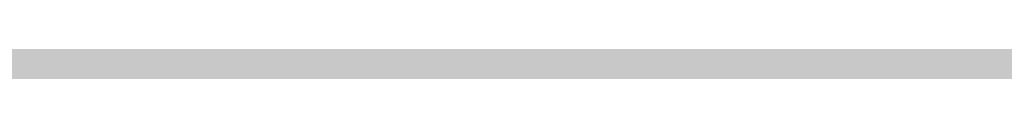
# Model space of a CAD drawing. Units: millimetres. Extents: x 0 to 2267, y 0 to 1823.
# Tile 151 of 256: x 1833.606 to 1838.83, y 1127.279 to 1127.355. Entities that reach past the tile are written whole.
import ezdxf

# ---------------------------------------------------------------- set-up
doc = ezdxf.new("R2010")
doc.units = ezdxf.units.MM
doc.header["$MEASUREMENT"] = 0
doc.layers.add('M-DIMS', color=2, linetype='Continuous', lineweight=25)
doc.layers.add('M-HATC', color=252, linetype='Continuous', lineweight=18)
doc.styles.get("Standard").update_dxf_attribs({"font": 'arial.ttf'})
doc.dimstyles.get("Standard").update_dxf_attribs({"dimtxt": 7, "dimasz": 4, "dimexe": 0.18, "dimexo": 0.0625, "dimgap": 0.09, "dimtad": 0, "dimdec": 0, "dimzin": 0, "dimdsep": 46, "dimtxsty": 'Standard', "dimcen": 0.09, "dimadec": 0, "dimazin": 0, "dimtfac": 1, "dimtdec": 0, "dimtofl": 0, "dimtmove": 0, "dimatfit": 3, "dimfxl": 1, "dimtolj": 1, "dimtzin": 0, "dimarcsym": 0})

# ---------------------------------------------------------------- blocks, each defined once
blk = doc.blocks.new('*D1')
at = {"layer": 'Defpoints', "color": 0, "transparency": 16777216}
for p in [(1593.4289, 1127.4171), (1843.4289, 1127.4171), (1843.4289, 955.6278)]:
    blk.add_point(p, dxfattribs=at)
at = {"layer": 'M-DIMS', "color": 0, "lineweight": -2, "transparency": 16777216}
for p, q in [((1593.4289, 1127.3546), (1593.4289, 955.4478)), ((1843.4289, 1127.3546), (1843.4289, 955.4478)), ((1597.4289, 955.6278), (1710.5582, 955.6278)), ((1839.4289, 955.6278), (1726.2996, 955.6278))]:
    blk.add_line(p, q, dxfattribs=at)
at = {"layer": 'M-DIMS', "color": 0, "transparency": 16777216}
for points in [[(1597.4289, 956.2944), (1597.4289, 954.9611), (1593.4289, 955.6278)], [(1839.4289, 956.2944), (1839.4289, 954.9611), (1843.4289, 955.6278)]]:
    blk.add_solid(points, dxfattribs=at)
at = {"layer": 'M-DIMS', "color": 0, "transparency": 16777216, "insert": (1718.4289, 955.6278), "char_height": 7, "attachment_point": 5}
blk.add_mtext('\\A1;250', dxfattribs=at)

msp = doc.modelspace()

# ---------------------------------------------------------------- hatches: boundary and pattern name
at = {"layer": 'M-HATC'}
h = msp.add_hatch(color=256, dxfattribs=at)
h.dxf.hatch_style = 1
h.paths.add_polyline_path([(2055.771, 1603.062), (1381.0868, 1603.062), (1381.0868, 1598.062), (2055.771, 1598.062)])
h.paths.add_polyline_path([(2055.771, 1598.062), (1381.0868, 1598.062), (1381.0868, 1593.062), (2055.771, 1593.062)])
h.paths.add_polyline_path([(2051.3074, 1536.7609), (1385.5504, 1536.7609), (1385.5504, 1526.7609), (1387.5504, 1526.7609), (1388.5366, 1525.0528), (1385.3319, 1521.2335), (1385.3319, 1521.2226), (2050.2542, 1522.7491), (2048.3212, 1525.0528), (2049.3074, 1526.7609), (2051.3074, 1526.7609)])
edge = h.paths.add_edge_path()
edge.add_arc((1847.5345, 1379.1492), 135, 222.603061, 222.890851, ccw=False)
edge.add_line((1748.1663, 1287.7656), (1683.0921, 1287.7656))
edge.add_arc((1583.7239, 1379.1492), 135, 317.109149, 317.396939, ccw=False)
edge.add_arc((1678.9686, 1290.6707), 5, 222.8909, 317.1091, ccw=False)
edge.add_arc((1774.2133, 1379.1492), 135, 222.603061, 222.890851, ccw=False)
edge.add_line((1674.8451, 1287.7656), (1609.7709, 1287.7656))
edge.add_arc((1510.4027, 1379.1492), 135, 317.109149, 317.396939, ccw=False)
edge.add_arc((1605.6474, 1290.6707), 5, 222.8909, 317.1091, ccw=False)
edge.add_arc((1700.8921, 1379.1492), 135, 222.603061, 222.890851, ccw=False)
edge.add_line((1601.5239, 1287.7656), (1536.4497, 1287.7656))
edge.add_arc((1437.0815, 1379.1492), 135, 317.109149, 317.396939, ccw=False)
edge.add_arc((1532.3262, 1290.6707), 5, 222.8909, 317.1091, ccw=False)
edge.add_arc((1627.5709, 1379.1492), 135, 222.603061, 222.890851, ccw=False)
edge.add_line((1528.2027, 1287.7656), (1505.9289, 1287.7656))
edge.add_spline(control_points=[(1505.9289, 1287.7656), (1504.2622, 1287.7656), (1504.2622, 1282.7656), (1505.9289, 1282.7656)], knot_values=[0, 0, 0, 0, 5, 5, 5, 5], degree=3, periodic=0)
edge.add_line((1505.9289, 1282.7656), (1930.9289, 1282.7656))
edge.add_spline(control_points=[(1930.9289, 1282.7656), (1932.5956, 1282.7656), (1932.5956, 1287.7656), (1930.9289, 1287.7656)], knot_values=[0, 0, 0, 0, 5, 5, 5, 5], degree=3, periodic=0)
edge.add_line((1930.9289, 1287.7656), (1903.0557, 1287.7656))
edge.add_arc((1803.6875, 1379.1492), 135, 317.109149, 317.396939, ccw=False)
edge.add_arc((1898.9322, 1290.6707), 5, 222.8909, 317.1091, ccw=False)
edge.add_arc((1994.1769, 1379.1492), 135, 222.603061, 222.890851, ccw=False)
edge.add_line((1894.8087, 1287.7656), (1829.7345, 1287.7656))
edge.add_arc((1730.3663, 1379.1492), 135, 317.109149, 317.396939, ccw=False)
edge.add_arc((1825.611, 1290.6707), 5, 222.8909, 317.1091, ccw=False)
edge.add_arc((1920.8557, 1379.1492), 135, 222.603061, 222.890851, ccw=False)
edge.add_line((1821.4875, 1287.7656), (1756.4133, 1287.7656))
edge.add_arc((1657.0451, 1379.1492), 135, 317.109149, 317.396939, ccw=False)
edge.add_arc((1752.2898, 1290.6707), 5, 222.8909, 317.1091, ccw=False)
edge = h.paths.add_edge_path()
edge.add_spline(control_points=[(1843.4289, 1227.2475), (1845.0956, 1227.2475), (1845.0956, 1232.2475), (1843.4289, 1232.2475)], knot_values=[0, 0, 0, 0, 5, 5, 5, 5], degree=3, periodic=0)
edge.add_line((1843.4289, 1232.2475), (1593.4289, 1232.2475))
edge.add_spline(control_points=[(1593.4289, 1232.2475), (1591.7622, 1232.2475), (1591.7622, 1227.2475), (1593.4289, 1227.2475)], knot_values=[0, 0, 0, 0, 5, 5, 5, 5], degree=3, periodic=0)
edge.add_line((1593.4289, 1227.2475), (1843.4289, 1227.2475))
h.paths.add_polyline_path([(1905.9289, 1127.4171), (1530.9289, 1127.4171, 0.414214), (1520.9289, 1117.4171), (1530.9289, 1117.4171), (1915.9289, 1117.4171, 0.414214)])
edge = h.paths.add_edge_path()
edge.add_arc((1397.0858, 1498.4078), 12.7299, 90.78215, 190.87871, ccw=False)
edge.add_line((1396.912, 1511.1365), (1428.0097, 1511.3488))
edge.add_line((1428.0097, 1511.3488), (1433.0097, 1511.3488))
edge.add_line((1433.0097, 1511.3488), (1434.439, 1511.3488))
edge.add_arc((1419.474, 1498.0804), 20, 41.561, 74.08211)
edge.add_line((1424.9592, 1517.3135), (1399.9351, 1517.2561))
edge.add_spline(control_points=[(1399.9307, 1517.2561), (1399.884, 1517.2131), (1399.8328, 1517.1689), (1399.7774, 1517.1236)], knot_values=[11.567499, 11.567499, 11.567499, 11.567499, 11.814249, 11.814249, 11.814249, 11.814249], degree=3, periodic=0)
edge.add_spline(control_points=[(1399.6328, 1517.0099), (1399.5831, 1516.9721), (1399.5307, 1516.9338), (1399.4759, 1516.8947)], knot_values=[11.167718, 11.167718, 11.167718, 11.167718, 11.365188, 11.365188, 11.365188, 11.365188], degree=3, periodic=0)
edge.add_spline(control_points=[(1399.3398, 1516.8001), (1399.1514, 1516.6719), (1398.9384, 1516.5377), (1398.704, 1516.3994)], knot_values=[10.376405, 10.376405, 10.376405, 10.376405, 11.00994, 11.00994, 11.00994, 11.00994], degree=3, periodic=0)
edge.add_spline(control_points=[(1398.6572, 1516.3719), (1398.5789, 1516.326), (1398.4983, 1516.2797), (1398.4155, 1516.2331)], knot_values=[10.125175, 10.125175, 10.125175, 10.125175, 10.334406, 10.334406, 10.334406, 10.334406], degree=3, periodic=0)
edge.add_spline(control_points=[(1398.2642, 1516.1487), (1398.196, 1516.1111), (1398.1263, 1516.0732), (1398.0555, 1516.0351)], knot_values=[9.832246, 9.832246, 9.832246, 9.832246, 9.999658, 9.999658, 9.999658, 9.999658], degree=3, periodic=0)
edge.add_spline(control_points=[(1397.9987, 1516.0048), (1397.7312, 1515.8621), (1397.446, 1515.7171), (1397.1466, 1515.5714)], knot_values=[9.161808, 9.161808, 9.161808, 9.161808, 9.787769, 9.787769, 9.787769, 9.787769], degree=3, periodic=0)
edge.add_spline(control_points=[(1397.1466, 1515.5714), (1396.8418, 1515.423), (1396.5222, 1515.274), (1396.1914, 1515.1262)], knot_values=[8.524455, 8.524455, 8.524455, 8.524455, 9.161808, 9.161808, 9.161808, 9.161808], degree=3, periodic=0)
edge.add_spline(control_points=[(1396.0777, 1515.0756), (1395.9854, 1515.0348), (1395.8922, 1514.994), (1395.7983, 1514.9534)], knot_values=[8.275193, 8.275193, 8.275193, 8.275193, 8.451726, 8.451726, 8.451726, 8.451726], degree=3, periodic=0)
edge.add_spline(control_points=[(1395.6018, 1514.8691), (1395.4997, 1514.8257), (1395.3968, 1514.7824), (1395.2932, 1514.7394)], knot_values=[7.962917, 7.962917, 7.962917, 7.962917, 8.152764, 8.152764, 8.152764, 8.152764], degree=3, periodic=0)
edge.add_spline(control_points=[(1395.2116, 1514.7057), (1394.8278, 1514.5475), (1394.4345, 1514.3929), (1394.0364, 1514.2442)], knot_values=[7.21254, 7.21254, 7.21254, 7.21254, 7.913148, 7.913148, 7.913148, 7.913148], degree=3, periodic=0)
edge.add_spline(control_points=[(1394.0364, 1514.2442), (1393.7076, 1514.1214), (1393.3754, 1514.0027), (1393.0427, 1513.8895)], knot_values=[6.633733, 6.633733, 6.633733, 6.633733, 7.21254, 7.21254, 7.21254, 7.21254], degree=3, periodic=0)
edge.add_spline(control_points=[(1392.8214, 1513.815), (1392.7198, 1513.7812), (1392.6181, 1513.7479), (1392.5166, 1513.7152)], knot_values=[6.328796, 6.328796, 6.328796, 6.328796, 6.505493, 6.505493, 6.505493, 6.505493], degree=3, periodic=0)
edge.add_spline(control_points=[(1392.5166, 1513.7152), (1392.3187, 1513.6515), (1392.1212, 1513.59), (1391.9244, 1513.531)], knot_values=[5.984605, 5.984605, 5.984605, 5.984605, 6.328796, 6.328796, 6.328796, 6.328796], degree=3, periodic=0)
edge.add_spline(control_points=[(1391.7915, 1513.4915), (1391.3122, 1513.3501), (1390.8384, 1513.2239), (1390.3784, 1513.1171)], knot_values=[5.066697, 5.066697, 5.066697, 5.066697, 5.907055, 5.907055, 5.907055, 5.907055], degree=3, periodic=0)
edge.add_spline(control_points=[(1390.3784, 1513.1171), (1390.1797, 1513.071), (1389.9836, 1513.0284), (1389.7907, 1512.9899)], knot_values=[4.70367, 4.70367, 4.70367, 4.70367, 5.066695, 5.066695, 5.066695, 5.066695], degree=3, periodic=0)
edge.add_spline(control_points=[(1389.422, 1512.9204), (1389.2459, 1512.8892), (1389.0729, 1512.8617), (1388.9036, 1512.8381)], knot_values=[4.130571, 4.130571, 4.130571, 4.130571, 4.469816, 4.469816, 4.469816, 4.469816], degree=3, periodic=0)
edge.add_spline(control_points=[(1388.9036, 1512.8381), (1388.591, 1512.7946), (1388.2911, 1512.7644), (1388.0071, 1512.7494)], knot_values=[3.504031, 3.504031, 3.504031, 3.504031, 4.130571, 4.130571, 4.130571, 4.130571], degree=3, periodic=0)
edge.add_spline(control_points=[(1387.9356, 1512.7459), (1387.8538, 1512.7423), (1387.7733, 1512.74), (1387.6944, 1512.739)], knot_values=[3.268866, 3.268866, 3.268866, 3.268866, 3.451164, 3.451164, 3.451164, 3.451164], degree=3, periodic=0)
edge.add_spline(control_points=[(1387.3351, 1512.7443), (1387.2076, 1512.7499), (1387.0847, 1512.7597), (1386.967, 1512.7739)], knot_values=[2.670686, 2.670686, 2.670686, 2.670686, 2.984, 2.984, 2.984, 2.984], degree=3, periodic=0)
edge.add_spline(control_points=[(1386.8327, 1512.7922), (1386.8209, 1512.7941), (1386.8092, 1512.7959), (1386.7975, 1512.7979)], knot_values=[2.516981, 2.516981, 2.516981, 2.516981, 2.549528, 2.549528, 2.549528, 2.549528], degree=3, periodic=0)
edge.add_spline(control_points=[(1386.4526, 1512.8735), (1386.4257, 1512.881), (1386.3993, 1512.889), (1386.3733, 1512.8972)], knot_values=[2.095869, 2.095869, 2.095869, 2.095869, 2.17941, 2.17941, 2.17941, 2.17941], degree=3, periodic=0)
edge.add_spline(control_points=[(1386.0691, 1513.0189), (1386.0634, 1513.0217), (1386.0577, 1513.0246), (1386.052, 1513.0275)], knot_values=[1.72453, 1.72453, 1.72453, 1.72453, 1.745933, 1.745933, 1.745933, 1.745933], degree=3, periodic=0)
edge.add_arc((1399.474, 1498.0804), 20, 131.82432, 180)
edge.add_arc((1630.3336, 1505.5484), 250.9708, 181.705176, 236.427975)
edge.add_arc((1605.3399, 1483.3044), 218.7822, 238.660829, 243.34961)
edge.add_arc((1647.0911, 1510.3592), 262.8986, 183.129836, 237.853442, ccw=False)
h.paths.add_polyline_path([(1406.5369, 1391.9644, 0.149382), (1491.5506, 1296.4418, -0.129517)], flags=17)
edge = h.paths.add_edge_path()
edge.add_arc((2037.3838, 1498.0804), 20, 0, 48.26587)
edge.add_spline(control_points=[(2050.6973, 1513.0052), (2050.6512, 1512.9847), (2050.6034, 1512.9655), (2050.5539, 1512.9477)], knot_values=[1.835652, 1.835652, 1.835652, 1.835652, 2.000781, 2.000781, 2.000781, 2.000781], degree=3, periodic=0)
edge.add_spline(control_points=[(2050.4616, 1512.9166), (2050.479, 1512.9221), (2050.4963, 1512.9277), (2050.5133, 1512.9335)], knot_values=[2.045477, 2.045477, 2.045477, 2.045477, 2.101389, 2.101389, 2.101389, 2.101389], degree=3, periodic=0)
edge.add_spline(control_points=[(2050.129, 1512.8342), (2050.1984, 1512.8473), (2050.2657, 1512.8623), (2050.3308, 1512.8792)], knot_values=[2.237629, 2.237629, 2.237629, 2.237629, 2.435841, 2.435841, 2.435841, 2.435841], degree=3, periodic=0)
edge.add_spline(control_points=[(2050.0946, 1512.8278), (2050.1061, 1512.8299), (2050.1176, 1512.832), (2050.129, 1512.8342)], knot_values=[2.435841, 2.435841, 2.435841, 2.435841, 2.468321, 2.468321, 2.468321, 2.468321], degree=3, periodic=0)
edge.add_spline(control_points=[(2049.7843, 1512.7851), (2049.8552, 1512.7922), (2049.9243, 1512.8008), (2049.9917, 1512.8109)], knot_values=[2.563852, 2.563852, 2.563852, 2.563852, 2.748541, 2.748541, 2.748541, 2.748541], degree=3, periodic=0)
edge.add_spline(control_points=[(2049.4052, 1512.7617), (2049.5364, 1512.7653), (2049.6629, 1512.773), (2049.7843, 1512.7851)], knot_values=[2.748541, 2.748541, 2.748541, 2.748541, 3.064882, 3.064882, 3.064882, 3.064882], degree=3, periodic=0)
edge.add_spline(control_points=[(2049.1698, 1512.7597), (2049.2336, 1512.7591), (2049.2965, 1512.7594), (2049.3584, 1512.7606)], knot_values=[3.102309, 3.102309, 3.102309, 3.102309, 3.2503, 3.2503, 3.2503, 3.2503], degree=3, periodic=0)
edge.add_spline(control_points=[(2048.8573, 1512.7691), (2048.9638, 1512.7638), (2049.068, 1512.7606), (2049.1698, 1512.7597)], knot_values=[3.2503, 3.2503, 3.2503, 3.2503, 3.486069, 3.486069, 3.486069, 3.486069], degree=3, periodic=0)
edge.add_spline(control_points=[(2048.6924, 1512.7789), (2048.3729, 1512.8009), (2048.0345, 1512.8411), (2047.6817, 1512.897)], knot_values=[3.606429, 3.606429, 3.606429, 3.606429, 4.2989, 4.2989, 4.2989, 4.2989], degree=3, periodic=0)
edge.add_spline(control_points=[(2047.6817, 1512.897), (2047.5458, 1512.9185), (2047.4077, 1512.9424), (2047.2678, 1512.9685)], knot_values=[4.2989, 4.2989, 4.2989, 4.2989, 4.565769, 4.565769, 4.565769, 4.565769], degree=3, periodic=0)
edge.add_spline(control_points=[(2047.2678, 1512.9685), (2047.1449, 1512.9914), (2047.0207, 1513.016), (2046.8951, 1513.0422)], knot_values=[4.565769, 4.565769, 4.565769, 4.565769, 4.799971, 4.799971, 4.799971, 4.799971], degree=3, periodic=0)
edge.add_spline(control_points=[(2046.8951, 1513.0422), (2046.5286, 1513.1188), (2046.1513, 1513.209), (2045.7676, 1513.3107)], knot_values=[4.799971, 4.799971, 4.799971, 4.799971, 5.483718, 5.483718, 5.483718, 5.483718], degree=3, periodic=0)
edge.add_spline(control_points=[(2045.7676, 1513.3107), (2045.3724, 1513.4154), (2044.9704, 1513.5322), (2044.5662, 1513.6588)], knot_values=[5.483718, 5.483718, 5.483718, 5.483718, 6.187866, 6.187866, 6.187866, 6.187866], degree=3, periodic=0)
edge.add_spline(control_points=[(2044.5662, 1513.6588), (2044.4149, 1513.7061), (2044.2633, 1513.7549), (2044.1116, 1513.8048)], knot_values=[6.187866, 6.187866, 6.187866, 6.187866, 6.451551, 6.451551, 6.451551, 6.451551], degree=3, periodic=0)
edge.add_spline(control_points=[(2044.1116, 1513.8048), (2043.9967, 1513.8427), (2043.8817, 1513.8813), (2043.7668, 1513.9205)], knot_values=[6.451551, 6.451551, 6.451551, 6.451551, 6.651434, 6.651434, 6.651434, 6.651434], degree=3, periodic=0)
edge.add_spline(control_points=[(2043.7668, 1513.9205), (2043.3716, 1514.0554), (2042.9774, 1514.1979), (2042.5886, 1514.3458)], knot_values=[6.651434, 6.651434, 6.651434, 6.651434, 7.338879, 7.338879, 7.338879, 7.338879], degree=3, periodic=0)
edge.add_spline(control_points=[(2042.5886, 1514.3458), (2042.1643, 1514.5071), (2041.7465, 1514.6749), (2041.3409, 1514.846)], knot_values=[7.338879, 7.338879, 7.338879, 7.338879, 8.089209, 8.089209, 8.089209, 8.089209], degree=3, periodic=0)
edge.add_spline(control_points=[(2041.3409, 1514.846), (2041.1028, 1514.9465), (2040.869, 1515.0481), (2040.6405, 1515.1502)], knot_values=[8.089209, 8.089209, 8.089209, 8.089209, 8.529587, 8.529587, 8.529587, 8.529587], degree=3, periodic=0)
edge.add_spline(control_points=[(2040.51, 1515.2089), (2040.0824, 1515.4022), (2039.6747, 1515.5971), (2039.295, 1515.7894)], knot_values=[8.613818, 8.613818, 8.613818, 8.613818, 9.44571, 9.44571, 9.44571, 9.44571], degree=3, periodic=0)
edge.add_spline(control_points=[(2039.295, 1515.7894), (2039.0618, 1515.9075), (2038.8391, 1516.0246), (2038.6288, 1516.1398)], knot_values=[9.44571, 9.44571, 9.44571, 9.44571, 9.956404, 9.956404, 9.956404, 9.956404], degree=3, periodic=0)
edge.add_spline(control_points=[(2038.6288, 1516.1398), (2038.5187, 1516.2001), (2038.4121, 1516.2598), (2038.309, 1516.3189)], knot_values=[9.956404, 9.956404, 9.956404, 9.956404, 10.223542, 10.223542, 10.223542, 10.223542], degree=3, periodic=0)
edge.add_spline(control_points=[(2038.309, 1516.3189), (2038.2138, 1516.3735), (2038.1216, 1516.4276), (2038.0328, 1516.481)], knot_values=[10.223542, 10.223542, 10.223542, 10.223542, 10.47051, 10.47051, 10.47051, 10.47051], degree=3, periodic=0)
edge.add_spline(control_points=[(2038.0328, 1516.481), (2037.7855, 1516.6296), (2037.5639, 1516.773), (2037.3722, 1516.909)], knot_values=[10.47051, 10.47051, 10.47051, 10.47051, 11.15767, 11.15767, 11.15767, 11.15767], degree=3, periodic=0)
edge.add_spline(control_points=[(2037.3722, 1516.909), (2037.2789, 1516.9752), (2037.1927, 1517.0396), (2037.1142, 1517.102)], knot_values=[11.15767, 11.15767, 11.15767, 11.15767, 11.49227, 11.49227, 11.49227, 11.49227], degree=3, periodic=0)
edge.add_spline(control_points=[(2036.8564, 1517.3259), (2036.9148, 1517.2692), (2036.9814, 1517.2103), (2037.0557, 1517.1492)], knot_values=[11.577341, 11.577341, 11.577341, 11.577341, 11.91035, 11.91035, 11.91035, 11.91035], degree=3, periodic=0)
edge.add_spline(control_points=[(2036.8074, 1517.3748), (2036.823, 1517.3587), (2036.8393, 1517.3424), (2036.8564, 1517.3259)], knot_values=[11.91035, 11.91035, 11.91035, 11.91035, 12.007402, 12.007402, 12.007402, 12.007402], degree=3, periodic=0)
edge.add_spline(control_points=[(2036.7017, 1517.494), (2036.7104, 1517.483), (2036.7196, 1517.4719), (2036.7291, 1517.4606)], knot_values=[12.184155, 12.184155, 12.184155, 12.184155, 12.255409, 12.255409, 12.255409, 12.255409], degree=3, periodic=0)
edge.add_spline(control_points=[(2036.6159, 1517.6205), (2036.62, 1517.613), (2036.6243, 1517.6055), (2036.6289, 1517.5979)], knot_values=[12.487913, 12.487913, 12.487913, 12.487913, 12.541035, 12.541035, 12.541035, 12.541035], degree=3, periodic=0)
edge.add_spline(control_points=[(2036.5635, 1517.786), (2036.5637, 1517.7794), (2036.5642, 1517.7726), (2036.565, 1517.7658)], knot_values=[12.911761, 12.911761, 12.911761, 12.911761, 12.968286, 12.968286, 12.968286, 12.968286], degree=3, periodic=0)
edge.add_spline(control_points=[(2036.6166, 1517.9304), (2036.6125, 1517.9259), (2036.6086, 1517.9212), (2036.6049, 1517.9165)], knot_values=[13.382527, 13.382527, 13.382527, 13.382527, 13.433791, 13.433791, 13.433791, 13.433791], degree=3, periodic=0)
edge.add_spline(control_points=[(2036.749, 1518.017), (2036.7361, 1518.0116), (2036.7239, 1518.006), (2036.7124, 1518.0002)], knot_values=[13.726299, 13.726299, 13.726299, 13.726299, 13.809928, 13.809928, 13.809928, 13.809928], degree=3, periodic=0)
edge.add_spline(control_points=[(2036.8604, 1518.0528), (2036.8386, 1518.0474), (2036.8181, 1518.0416), (2036.7988, 1518.0353)], knot_values=[13.910887, 13.910887, 13.910887, 13.910887, 14.02153, 14.02153, 14.02153, 14.02153], degree=3, periodic=0)
edge.add_line((2036.9639, 1518.0804), (2032.3838, 1518.0804))
edge.add_line((2032.3838, 1518.0804), (2027.3838, 1518.0804))
edge.add_line((2027.3838, 1518.0804), (2022.3838, 1518.0804))
edge.add_line((2022.3838, 1518.0804), (2017.3838, 1518.0804))
edge.add_arc((2017.3838, 1498.0804), 20, 90, 138.439)
edge.add_line((2002.4188, 1511.3488), (2003.8481, 1511.3488))
edge.add_line((2003.8481, 1511.3488), (2008.8481, 1511.3488))
edge.add_line((2008.8481, 1511.3488), (2039.772, 1511.1377))
edge.add_arc((2039.772, 1498.4078), 12.7299, -10.87871, 90, ccw=False)
edge.add_arc((1789.7668, 1510.3592), 262.8986, 302.146558, 356.870164, ccw=False)
edge.add_arc((1831.5179, 1483.3044), 218.7822, 296.65039, 301.339171)
edge.add_arc((1806.5242, 1505.5484), 250.9708, 303.572025, 358.294824)
h.paths.add_polyline_path([(2030.321, 1391.9644, -0.129517), (1945.3072, 1296.4418, 0.149382)], flags=17)
edge = h.paths.add_edge_path()
edge.add_spline(control_points=[(2037.2464, 1518.0821), (2037.2898, 1518.081), (2037.3355, 1518.0804), (2037.3838, 1518.0804)], knot_values=[0.000012, 0.000012, 0.000012, 0.000012, 0.144754, 0.144754, 0.144754, 0.144754], degree=3, periodic=0)
edge.add_line((2037.3357, 1518.0804), (2037.0096, 1518.0804))
edge.add_spline(control_points=[(2037.0096, 1518.0804), (2036.9822, 1518.0768), (2036.956, 1518.0727), (2036.9312, 1518.0681)], knot_values=[14.13465, 14.13465, 14.13465, 14.13465, 14.247197, 14.247197, 14.247197, 14.247197], degree=3, periodic=0)
edge.add_spline(control_points=[(2036.9312, 1518.0681), (2036.9276, 1518.0674), (2036.9241, 1518.0667), (2036.9205, 1518.0661)], knot_values=[14.118315, 14.118315, 14.118315, 14.118315, 14.13465, 14.13465, 14.13465, 14.13465], degree=3, periodic=0)
edge.add_spline(control_points=[(2036.9205, 1518.0661), (2036.9118, 1518.0644), (2036.9032, 1518.0626), (2036.8948, 1518.0608)], knot_values=[14.078086, 14.078086, 14.078086, 14.078086, 14.118315, 14.118315, 14.118315, 14.118315], degree=3, periodic=0)
edge.add_spline(control_points=[(2036.8948, 1518.0608), (2036.883, 1518.0583), (2036.8716, 1518.0556), (2036.8604, 1518.0528)], knot_values=[14.02153, 14.02153, 14.02153, 14.02153, 14.078086, 14.078086, 14.078086, 14.078086], degree=3, periodic=0)
edge.add_spline(control_points=[(2036.8604, 1518.0528), (2036.8386, 1518.0474), (2036.8181, 1518.0416), (2036.7988, 1518.0353)], knot_values=[13.910887, 13.910887, 13.910887, 13.910887, 14.02153, 14.02153, 14.02153, 14.02153], degree=3, periodic=0)
edge.add_spline(control_points=[(2036.7988, 1518.0353), (2036.7981, 1518.035), (2036.7974, 1518.0348), (2036.7967, 1518.0346)], knot_values=[13.906906, 13.906906, 13.906906, 13.906906, 13.910887, 13.910887, 13.910887, 13.910887], degree=3, periodic=0)
edge.add_spline(control_points=[(2036.7967, 1518.0346), (2036.7882, 1518.0318), (2036.7799, 1518.0289), (2036.7719, 1518.0259)], knot_values=[13.857826, 13.857826, 13.857826, 13.857826, 13.906906, 13.906906, 13.906906, 13.906906], degree=3, periodic=0)
edge.add_spline(control_points=[(2036.7719, 1518.0259), (2036.764, 1518.023), (2036.7564, 1518.02), (2036.749, 1518.017)], knot_values=[13.809928, 13.809928, 13.809928, 13.809928, 13.857826, 13.857826, 13.857826, 13.857826], degree=3, periodic=0)
edge.add_spline(control_points=[(2036.749, 1518.017), (2036.7361, 1518.0116), (2036.7239, 1518.006), (2036.7124, 1518.0002)], knot_values=[13.726299, 13.726299, 13.726299, 13.726299, 13.809928, 13.809928, 13.809928, 13.809928], degree=3, periodic=0)
edge.add_spline(control_points=[(2036.7124, 1518.0002), (2036.7121, 1518), (2036.7118, 1517.9999), (2036.7115, 1517.9997)], knot_values=[13.723993, 13.723993, 13.723993, 13.723993, 13.726299, 13.726299, 13.726299, 13.726299], degree=3, periodic=0)
edge.add_spline(control_points=[(2036.7115, 1517.9997), (2036.7063, 1517.9971), (2036.7013, 1517.9944), (2036.6965, 1517.9917)], knot_values=[13.686536, 13.686536, 13.686536, 13.686536, 13.723993, 13.723993, 13.723993, 13.723993], degree=3, periodic=0)
edge.add_spline(control_points=[(2036.6965, 1517.9917), (2036.6919, 1517.9891), (2036.6874, 1517.9865), (2036.6831, 1517.9839)], knot_values=[13.651251, 13.651251, 13.651251, 13.651251, 13.686536, 13.686536, 13.686536, 13.686536], degree=3, periodic=0)
edge.add_spline(control_points=[(2036.6831, 1517.9839), (2036.6764, 1517.9798), (2036.67, 1517.9757), (2036.6639, 1517.9714)], knot_values=[13.596804, 13.596804, 13.596804, 13.596804, 13.651251, 13.651251, 13.651251, 13.651251], degree=3, periodic=0)
edge.add_spline(control_points=[(2036.6639, 1517.9714), (2036.6636, 1517.9712), (2036.6633, 1517.9709), (2036.6629, 1517.9707)], knot_values=[13.593956, 13.593956, 13.593956, 13.593956, 13.596804, 13.596804, 13.596804, 13.596804], degree=3, periodic=0)
edge.add_spline(control_points=[(2036.6629, 1517.9707), (2036.6603, 1517.9689), (2036.6577, 1517.967), (2036.6552, 1517.9651)], knot_values=[13.570322, 13.570322, 13.570322, 13.570322, 13.593956, 13.593956, 13.593956, 13.593956], degree=3, periodic=0)
edge.add_spline(control_points=[(2036.6552, 1517.9651), (2036.6525, 1517.9631), (2036.6499, 1517.9611), (2036.6474, 1517.9591)], knot_values=[13.545477, 13.545477, 13.545477, 13.545477, 13.570322, 13.570322, 13.570322, 13.570322], degree=3, periodic=0)
edge.add_spline(control_points=[(2036.6474, 1517.9591), (2036.6472, 1517.9589), (2036.6471, 1517.9588), (2036.6469, 1517.9587)], knot_values=[13.543931, 13.543931, 13.543931, 13.543931, 13.545477, 13.545477, 13.545477, 13.545477], degree=3, periodic=0)
edge.add_spline(control_points=[(2036.6469, 1517.9587), (2036.6412, 1517.9541), (2036.6358, 1517.9494), (2036.6307, 1517.9447)], knot_values=[13.488237, 13.488237, 13.488237, 13.488237, 13.543931, 13.543931, 13.543931, 13.543931], degree=3, periodic=0)
edge.add_spline(control_points=[(2036.6307, 1517.9447), (2036.6282, 1517.9423), (2036.6257, 1517.9399), (2036.6233, 1517.9374)], knot_values=[13.460307, 13.460307, 13.460307, 13.460307, 13.488237, 13.488237, 13.488237, 13.488237], degree=3, periodic=0)
edge.add_spline(control_points=[(2036.6233, 1517.9374), (2036.6215, 1517.9356), (2036.6198, 1517.9338), (2036.6181, 1517.932)], knot_values=[13.439712, 13.439712, 13.439712, 13.439712, 13.460307, 13.460307, 13.460307, 13.460307], degree=3, periodic=0)
edge.add_spline(control_points=[(2036.6181, 1517.932), (2036.6176, 1517.9315), (2036.6171, 1517.9309), (2036.6166, 1517.9304)], knot_values=[13.433791, 13.433791, 13.433791, 13.433791, 13.439712, 13.439712, 13.439712, 13.439712], degree=3, periodic=0)
edge.add_spline(control_points=[(2036.6166, 1517.9304), (2036.6125, 1517.9259), (2036.6086, 1517.9212), (2036.6049, 1517.9165)], knot_values=[13.382527, 13.382527, 13.382527, 13.382527, 13.433791, 13.433791, 13.433791, 13.433791], degree=3, periodic=0)
edge.add_spline(control_points=[(2036.6049, 1517.9165), (2036.6026, 1517.9135), (2036.6004, 1517.9104), (2036.5982, 1517.9074)], knot_values=[13.350017, 13.350017, 13.350017, 13.350017, 13.382527, 13.382527, 13.382527, 13.382527], degree=3, periodic=0)
edge.add_spline(control_points=[(2036.5982, 1517.9074), (2036.5972, 1517.9059), (2036.5962, 1517.9043), (2036.5952, 1517.9028)], knot_values=[13.333922, 13.333922, 13.333922, 13.333922, 13.350017, 13.350017, 13.350017, 13.350017], degree=3, periodic=0)
edge.add_spline(control_points=[(2036.5952, 1517.9028), (2036.5945, 1517.9018), (2036.5939, 1517.9009), (2036.5933, 1517.8999)], knot_values=[13.323828, 13.323828, 13.323828, 13.323828, 13.333922, 13.333922, 13.333922, 13.333922], degree=3, periodic=0)
edge.add_spline(control_points=[(2036.5933, 1517.8999), (2036.5905, 1517.8955), (2036.5879, 1517.8909), (2036.5855, 1517.8864)], knot_values=[13.277545, 13.277545, 13.277545, 13.277545, 13.323828, 13.323828, 13.323828, 13.323828], degree=3, periodic=0)
edge.add_spline(control_points=[(2036.5855, 1517.8864), (2036.5836, 1517.8827), (2036.5817, 1517.8789), (2036.5801, 1517.8751)], knot_values=[13.240119, 13.240119, 13.240119, 13.240119, 13.277545, 13.277545, 13.277545, 13.277545], degree=3, periodic=0)
edge.add_spline(control_points=[(2036.5801, 1517.8751), (2036.5795, 1517.8739), (2036.579, 1517.8727), (2036.5785, 1517.8715)], knot_values=[13.228211, 13.228211, 13.228211, 13.228211, 13.240119, 13.240119, 13.240119, 13.240119], degree=3, periodic=0)
edge.add_spline(control_points=[(2036.5785, 1517.8715), (2036.578, 1517.8702), (2036.5774, 1517.869), (2036.5769, 1517.8677)], knot_values=[13.215717, 13.215717, 13.215717, 13.215717, 13.228211, 13.228211, 13.228211, 13.228211], degree=3, periodic=0)
edge.add_spline(control_points=[(2036.5769, 1517.8677), (2036.5755, 1517.864), (2036.5741, 1517.8603), (2036.5729, 1517.8565)], knot_values=[13.179847, 13.179847, 13.179847, 13.179847, 13.215717, 13.215717, 13.215717, 13.215717], degree=3, periodic=0)
edge.add_spline(control_points=[(2036.5729, 1517.8565), (2036.5713, 1517.8515), (2036.5699, 1517.8464), (2036.5687, 1517.8413)], knot_values=[13.132017, 13.132017, 13.132017, 13.132017, 13.179847, 13.179847, 13.179847, 13.179847], degree=3, periodic=0)
edge.add_spline(control_points=[(2036.5687, 1517.8413), (2036.5684, 1517.8402), (2036.5682, 1517.8392), (2036.568, 1517.8382)], knot_values=[13.122482, 13.122482, 13.122482, 13.122482, 13.132017, 13.132017, 13.132017, 13.132017], degree=3, periodic=0)
edge.add_spline(control_points=[(2036.568, 1517.8382), (2036.5676, 1517.8363), (2036.5672, 1517.8345), (2036.5669, 1517.8327)], knot_values=[13.105592, 13.105592, 13.105592, 13.105592, 13.122482, 13.122482, 13.122482, 13.122482], degree=3, periodic=0)
edge.add_spline(control_points=[(2036.5669, 1517.8327), (2036.5662, 1517.8292), (2036.5657, 1517.8257), (2036.5652, 1517.8222)], knot_values=[13.074063, 13.074063, 13.074063, 13.074063, 13.105592, 13.105592, 13.105592, 13.105592], degree=3, periodic=0)
edge.add_spline(control_points=[(2036.5652, 1517.8222), (2036.5652, 1517.8222), (2036.5652, 1517.8222), (2036.5652, 1517.8222)], knot_values=[13.074043, 13.074043, 13.074043, 13.074043, 13.074063, 13.074063, 13.074063, 13.074063], degree=3, periodic=0)
edge.add_spline(control_points=[(2036.5652, 1517.8222), (2036.5644, 1517.8164), (2036.5639, 1517.8106), (2036.5636, 1517.8046)], knot_values=[13.021884, 13.021884, 13.021884, 13.021884, 13.074043, 13.074043, 13.074043, 13.074043], degree=3, periodic=0)
edge.add_spline(control_points=[(2036.5636, 1517.8046), (2036.5636, 1517.804), (2036.5636, 1517.8034), (2036.5635, 1517.8028)], knot_values=[13.01674, 13.01674, 13.01674, 13.01674, 13.021884, 13.021884, 13.021884, 13.021884], degree=3, periodic=0)
edge.add_spline(control_points=[(2036.5635, 1517.8028), (2036.5634, 1517.8005), (2036.5634, 1517.7982), (2036.5634, 1517.7958)], knot_values=[12.996438, 12.996438, 12.996438, 12.996438, 13.01674, 13.01674, 13.01674, 13.01674], degree=3, periodic=0)
edge.add_spline(control_points=[(2036.5634, 1517.7958), (2036.5633, 1517.7926), (2036.5634, 1517.7893), (2036.5635, 1517.786)], knot_values=[12.968286, 12.968286, 12.968286, 12.968286, 12.996438, 12.996438, 12.996438, 12.996438], degree=3, periodic=0)
edge.add_spline(control_points=[(2036.5635, 1517.786), (2036.5637, 1517.7794), (2036.5642, 1517.7726), (2036.565, 1517.7658)], knot_values=[12.911761, 12.911761, 12.911761, 12.911761, 12.968286, 12.968286, 12.968286, 12.968286], degree=3, periodic=0)
edge.add_spline(control_points=[(2036.565, 1517.7658), (2036.565, 1517.7657), (2036.565, 1517.7656), (2036.565, 1517.7656)], knot_values=[12.911017, 12.911017, 12.911017, 12.911017, 12.911761, 12.911761, 12.911761, 12.911761], degree=3, periodic=0)
edge.add_spline(control_points=[(2036.565, 1517.7656), (2036.5654, 1517.7625), (2036.5658, 1517.7593), (2036.5663, 1517.7562)], knot_values=[12.88528, 12.88528, 12.88528, 12.88528, 12.911017, 12.911017, 12.911017, 12.911017], degree=3, periodic=0)
edge.add_spline(control_points=[(2036.5663, 1517.7562), (2036.5667, 1517.7534), (2036.5672, 1517.7506), (2036.5677, 1517.7478)], knot_values=[12.862519, 12.862519, 12.862519, 12.862519, 12.88528, 12.88528, 12.88528, 12.88528], degree=3, periodic=0)
edge.add_spline(control_points=[(2036.5677, 1517.7478), (2036.5678, 1517.7474), (2036.5679, 1517.7469), (2036.568, 1517.7465)], knot_values=[12.858885, 12.858885, 12.858885, 12.858885, 12.862519, 12.862519, 12.862519, 12.862519], degree=3, periodic=0)
edge.add_spline(control_points=[(2036.568, 1517.7465), (2036.5692, 1517.7399), (2036.5707, 1517.7332), (2036.5724, 1517.7264)], knot_values=[12.8053, 12.8053, 12.8053, 12.8053, 12.858885, 12.858885, 12.858885, 12.858885], degree=3, periodic=0)
edge.add_spline(control_points=[(2036.5724, 1517.7264), (2036.5734, 1517.7226), (2036.5745, 1517.7187), (2036.5756, 1517.7149)], knot_values=[12.775176, 12.775176, 12.775176, 12.775176, 12.8053, 12.8053, 12.8053, 12.8053], degree=3, periodic=0)
edge.add_spline(control_points=[(2036.5756, 1517.7149), (2036.5763, 1517.7125), (2036.577, 1517.7102), (2036.5778, 1517.7078)], knot_values=[12.756759, 12.756759, 12.756759, 12.756759, 12.775176, 12.775176, 12.775176, 12.775176], degree=3, periodic=0)
edge.add_spline(control_points=[(2036.5778, 1517.7078), (2036.5781, 1517.7067), (2036.5784, 1517.7057), (2036.5787, 1517.7047)], knot_values=[12.748742, 12.748742, 12.748742, 12.748742, 12.756759, 12.756759, 12.756759, 12.756759], degree=3, periodic=0)
edge.add_spline(control_points=[(2036.5787, 1517.7047), (2036.5808, 1517.6983), (2036.5831, 1517.6919), (2036.5856, 1517.6854)], knot_values=[12.69959, 12.69959, 12.69959, 12.69959, 12.748742, 12.748742, 12.748742, 12.748742], degree=3, periodic=0)
edge.add_spline(control_points=[(2036.5856, 1517.6854), (2036.5876, 1517.68), (2036.5898, 1517.6746), (2036.5921, 1517.6692)], knot_values=[12.659038, 12.659038, 12.659038, 12.659038, 12.69959, 12.69959, 12.69959, 12.69959], degree=3, periodic=0)
edge.add_spline(control_points=[(2036.5921, 1517.6692), (2036.594, 1517.6648), (2036.5959, 1517.6605), (2036.5979, 1517.6561)], knot_values=[12.626806, 12.626806, 12.626806, 12.626806, 12.659038, 12.659038, 12.659038, 12.659038], degree=3, periodic=0)
edge.add_spline(control_points=[(2036.5979, 1517.6561), (2036.5984, 1517.6551), (2036.5989, 1517.6541), (2036.5993, 1517.6531)], knot_values=[12.619394, 12.619394, 12.619394, 12.619394, 12.626806, 12.626806, 12.626806, 12.626806], degree=3, periodic=0)
edge.add_spline(control_points=[(2036.5993, 1517.6531), (2036.6043, 1517.6424), (2036.6099, 1517.6315), (2036.6159, 1517.6205)], knot_values=[12.541039, 12.541039, 12.541039, 12.541039, 12.619394, 12.619394, 12.619394, 12.619394], degree=3, periodic=0)
edge.add_spline(control_points=[(2036.6159, 1517.6205), (2036.6159, 1517.6205), (2036.6159, 1517.6205), (2036.6159, 1517.6205)], knot_values=[12.541035, 12.541035, 12.541035, 12.541035, 12.541039, 12.541039, 12.541039, 12.541039], degree=3, periodic=0)
edge.add_spline(control_points=[(2036.6159, 1517.6205), (2036.62, 1517.613), (2036.6243, 1517.6055), (2036.6289, 1517.5979)], knot_values=[12.487913, 12.487913, 12.487913, 12.487913, 12.541035, 12.541035, 12.541035, 12.541035], degree=3, periodic=0)
edge.add_spline(control_points=[(2036.6289, 1517.5979), (2036.6326, 1517.5916), (2036.6365, 1517.5853), (2036.6406, 1517.5789)], knot_values=[12.443982, 12.443982, 12.443982, 12.443982, 12.487913, 12.487913, 12.487913, 12.487913], degree=3, periodic=0)
edge.add_spline(control_points=[(2036.6406, 1517.5789), (2036.6414, 1517.5776), (2036.6423, 1517.5763), (2036.6431, 1517.5749)], knot_values=[12.434996, 12.434996, 12.434996, 12.434996, 12.443982, 12.443982, 12.443982, 12.443982], degree=3, periodic=0)
edge.add_spline(control_points=[(2036.6431, 1517.5749), (2036.6531, 1517.5596), (2036.6639, 1517.5439), (2036.6756, 1517.528)], knot_values=[12.329647, 12.329647, 12.329647, 12.329647, 12.434996, 12.434996, 12.434996, 12.434996], degree=3, periodic=0)
edge.add_spline(control_points=[(2036.6756, 1517.528), (2036.6839, 1517.5168), (2036.6925, 1517.5055), (2036.7017, 1517.494)], knot_values=[12.255409, 12.255409, 12.255409, 12.255409, 12.329647, 12.329647, 12.329647, 12.329647], degree=3, periodic=0)
edge.add_spline(control_points=[(2036.7017, 1517.494), (2036.7104, 1517.483), (2036.7196, 1517.4719), (2036.7291, 1517.4606)], knot_values=[12.184155, 12.184155, 12.184155, 12.184155, 12.255409, 12.255409, 12.255409, 12.255409], degree=3, periodic=0)
edge.add_spline(control_points=[(2036.7291, 1517.4606), (2036.7436, 1517.4435), (2036.759, 1517.4262), (2036.7753, 1517.4085)], knot_values=[12.075961, 12.075961, 12.075961, 12.075961, 12.184155, 12.184155, 12.184155, 12.184155], degree=3, periodic=0)
edge.add_spline(control_points=[(2036.7753, 1517.4085), (2036.7763, 1517.4075), (2036.7773, 1517.4064), (2036.7783, 1517.4054)], knot_values=[12.069502, 12.069502, 12.069502, 12.069502, 12.075961, 12.075961, 12.075961, 12.075961], degree=3, periodic=0)
edge.add_spline(control_points=[(2036.7783, 1517.4054), (2036.7877, 1517.3953), (2036.7974, 1517.385), (2036.8074, 1517.3748)], knot_values=[12.007402, 12.007402, 12.007402, 12.007402, 12.069502, 12.069502, 12.069502, 12.069502], degree=3, periodic=0)
edge.add_spline(control_points=[(2036.8074, 1517.3748), (2036.823, 1517.3587), (2036.8393, 1517.3424), (2036.8564, 1517.3259)], knot_values=[11.91035, 11.91035, 11.91035, 11.91035, 12.007402, 12.007402, 12.007402, 12.007402], degree=3, periodic=0)
edge.add_spline(control_points=[(2036.8564, 1517.3259), (2036.9148, 1517.2692), (2036.9814, 1517.2103), (2037.0557, 1517.1492)], knot_values=[11.577341, 11.577341, 11.577341, 11.577341, 11.91035, 11.91035, 11.91035, 11.91035], degree=3, periodic=0)
edge.add_spline(control_points=[(2037.0557, 1517.1492), (2037.0747, 1517.1336), (2037.0942, 1517.1179), (2037.1142, 1517.102)], knot_values=[11.49227, 11.49227, 11.49227, 11.49227, 11.577341, 11.577341, 11.577341, 11.577341], degree=3, periodic=0)
edge.add_spline(control_points=[(2037.1142, 1517.102), (2037.1927, 1517.0396), (2037.2789, 1516.9752), (2037.3722, 1516.909)], knot_values=[11.15767, 11.15767, 11.15767, 11.15767, 11.49227, 11.49227, 11.49227, 11.49227], degree=3, periodic=0)
edge.add_spline(control_points=[(2037.3722, 1516.909), (2037.5639, 1516.773), (2037.7855, 1516.6296), (2038.0328, 1516.481)], knot_values=[10.47051, 10.47051, 10.47051, 10.47051, 11.15767, 11.15767, 11.15767, 11.15767], degree=3, periodic=0)
edge.add_spline(control_points=[(2038.0328, 1516.481), (2038.1216, 1516.4276), (2038.2138, 1516.3735), (2038.309, 1516.3189)], knot_values=[10.223542, 10.223542, 10.223542, 10.223542, 10.47051, 10.47051, 10.47051, 10.47051], degree=3, periodic=0)
edge.add_spline(control_points=[(2038.309, 1516.3189), (2038.4121, 1516.2598), (2038.5187, 1516.2001), (2038.6288, 1516.1398)], knot_values=[9.956404, 9.956404, 9.956404, 9.956404, 10.223542, 10.223542, 10.223542, 10.223542], degree=3, periodic=0)
edge.add_spline(control_points=[(2038.6288, 1516.1398), (2038.8391, 1516.0246), (2039.0618, 1515.9075), (2039.295, 1515.7894)], knot_values=[9.44571, 9.44571, 9.44571, 9.44571, 9.956404, 9.956404, 9.956404, 9.956404], degree=3, periodic=0)
edge.add_spline(control_points=[(2039.295, 1515.7894), (2039.6747, 1515.5971), (2040.0824, 1515.4022), (2040.51, 1515.2089)], knot_values=[8.613818, 8.613818, 8.613818, 8.613818, 9.44571, 9.44571, 9.44571, 9.44571], degree=3, periodic=0)
edge.add_spline(control_points=[(2040.51, 1515.2089), (2040.5533, 1515.1893), (2040.5968, 1515.1697), (2040.6405, 1515.1502)], knot_values=[8.529587, 8.529587, 8.529587, 8.529587, 8.613818, 8.613818, 8.613818, 8.613818], degree=3, periodic=0)
edge.add_spline(control_points=[(2040.6405, 1515.1502), (2040.869, 1515.0481), (2041.1028, 1514.9465), (2041.3409, 1514.846)], knot_values=[8.089209, 8.089209, 8.089209, 8.089209, 8.529587, 8.529587, 8.529587, 8.529587], degree=3, periodic=0)
edge.add_spline(control_points=[(2041.3409, 1514.846), (2041.7465, 1514.6749), (2042.1643, 1514.5071), (2042.5886, 1514.3458)], knot_values=[7.338879, 7.338879, 7.338879, 7.338879, 8.089209, 8.089209, 8.089209, 8.089209], degree=3, periodic=0)
edge.add_spline(control_points=[(2042.5886, 1514.3458), (2042.9774, 1514.1979), (2043.3716, 1514.0554), (2043.7668, 1513.9205)], knot_values=[6.651434, 6.651434, 6.651434, 6.651434, 7.338879, 7.338879, 7.338879, 7.338879], degree=3, periodic=0)
edge.add_spline(control_points=[(2043.7668, 1513.9205), (2043.8817, 1513.8813), (2043.9967, 1513.8427), (2044.1116, 1513.8048)], knot_values=[6.451551, 6.451551, 6.451551, 6.451551, 6.651434, 6.651434, 6.651434, 6.651434], degree=3, periodic=0)
edge.add_spline(control_points=[(2044.1116, 1513.8048), (2044.2633, 1513.7549), (2044.4149, 1513.7061), (2044.5662, 1513.6588)], knot_values=[6.187866, 6.187866, 6.187866, 6.187866, 6.451551, 6.451551, 6.451551, 6.451551], degree=3, periodic=0)
edge.add_spline(control_points=[(2044.5662, 1513.6588), (2044.9704, 1513.5322), (2045.3724, 1513.4154), (2045.7676, 1513.3107)], knot_values=[5.483718, 5.483718, 5.483718, 5.483718, 6.187866, 6.187866, 6.187866, 6.187866], degree=3, periodic=0)
edge.add_spline(control_points=[(2045.7676, 1513.3107), (2046.1513, 1513.209), (2046.5286, 1513.1188), (2046.8951, 1513.0422)], knot_values=[4.799971, 4.799971, 4.799971, 4.799971, 5.483718, 5.483718, 5.483718, 5.483718], degree=3, periodic=0)
edge.add_spline(control_points=[(2046.8951, 1513.0422), (2047.0207, 1513.016), (2047.1449, 1512.9914), (2047.2678, 1512.9685)], knot_values=[4.565769, 4.565769, 4.565769, 4.565769, 4.799971, 4.799971, 4.799971, 4.799971], degree=3, periodic=0)
edge.add_spline(control_points=[(2047.2678, 1512.9685), (2047.4077, 1512.9424), (2047.5458, 1512.9185), (2047.6817, 1512.897)], knot_values=[4.2989, 4.2989, 4.2989, 4.2989, 4.565769, 4.565769, 4.565769, 4.565769], degree=3, periodic=0)
edge.add_spline(control_points=[(2047.6817, 1512.897), (2048.0345, 1512.8411), (2048.3729, 1512.8009), (2048.6924, 1512.7789)], knot_values=[3.606429, 3.606429, 3.606429, 3.606429, 4.2989, 4.2989, 4.2989, 4.2989], degree=3, periodic=0)
edge.add_spline(control_points=[(2048.6924, 1512.7789), (2048.7479, 1512.7751), (2048.8029, 1512.7718), (2048.8573, 1512.7691)], knot_values=[3.486069, 3.486069, 3.486069, 3.486069, 3.606429, 3.606429, 3.606429, 3.606429], degree=3, periodic=0)
edge.add_spline(control_points=[(2048.8573, 1512.7691), (2048.9638, 1512.7638), (2049.068, 1512.7606), (2049.1698, 1512.7597)], knot_values=[3.2503, 3.2503, 3.2503, 3.2503, 3.486069, 3.486069, 3.486069, 3.486069], degree=3, periodic=0)
edge.add_spline(control_points=[(2049.1698, 1512.7597), (2049.2336, 1512.7591), (2049.2965, 1512.7594), (2049.3584, 1512.7606)], knot_values=[3.102309, 3.102309, 3.102309, 3.102309, 3.2503, 3.2503, 3.2503, 3.2503], degree=3, periodic=0)
edge.add_spline(control_points=[(2049.3584, 1512.7606), (2049.3741, 1512.7609), (2049.3897, 1512.7613), (2049.4052, 1512.7617)], knot_values=[3.064882, 3.064882, 3.064882, 3.064882, 3.102309, 3.102309, 3.102309, 3.102309], degree=3, periodic=0)
edge.add_spline(control_points=[(2049.4052, 1512.7617), (2049.5364, 1512.7653), (2049.6629, 1512.773), (2049.7843, 1512.7851)], knot_values=[2.748541, 2.748541, 2.748541, 2.748541, 3.064882, 3.064882, 3.064882, 3.064882], degree=3, periodic=0)
edge.add_spline(control_points=[(2049.7843, 1512.7851), (2049.8552, 1512.7922), (2049.9243, 1512.8008), (2049.9917, 1512.8109)], knot_values=[2.563852, 2.563852, 2.563852, 2.563852, 2.748541, 2.748541, 2.748541, 2.748541], degree=3, periodic=0)
edge.add_spline(control_points=[(2049.9917, 1512.8109), (2050.0265, 1512.8161), (2050.0608, 1512.8218), (2050.0946, 1512.8278)], knot_values=[2.468321, 2.468321, 2.468321, 2.468321, 2.563852, 2.563852, 2.563852, 2.563852], degree=3, periodic=0)
edge.add_spline(control_points=[(2050.0946, 1512.8278), (2050.1061, 1512.8299), (2050.1176, 1512.832), (2050.129, 1512.8342)], knot_values=[2.435841, 2.435841, 2.435841, 2.435841, 2.468321, 2.468321, 2.468321, 2.468321], degree=3, periodic=0)
edge.add_spline(control_points=[(2050.129, 1512.8342), (2050.1984, 1512.8473), (2050.2657, 1512.8623), (2050.3308, 1512.8792)], knot_values=[2.237629, 2.237629, 2.237629, 2.237629, 2.435841, 2.435841, 2.435841, 2.435841], degree=3, periodic=0)
edge.add_spline(control_points=[(2050.3308, 1512.8792), (2050.3754, 1512.8908), (2050.4191, 1512.9032), (2050.4616, 1512.9166)], knot_values=[2.101389, 2.101389, 2.101389, 2.101389, 2.237629, 2.237629, 2.237629, 2.237629], degree=3, periodic=0)
edge.add_spline(control_points=[(2050.4616, 1512.9166), (2050.479, 1512.9221), (2050.4963, 1512.9277), (2050.5133, 1512.9335)], knot_values=[2.045477, 2.045477, 2.045477, 2.045477, 2.101389, 2.101389, 2.101389, 2.101389], degree=3, periodic=0)
edge.add_spline(control_points=[(2050.5133, 1512.9335), (2050.527, 1512.9382), (2050.5405, 1512.9429), (2050.5539, 1512.9477)], knot_values=[2.000781, 2.000781, 2.000781, 2.000781, 2.045477, 2.045477, 2.045477, 2.045477], degree=3, periodic=0)
edge.add_spline(control_points=[(2050.5539, 1512.9477), (2050.6034, 1512.9655), (2050.6512, 1512.9847), (2050.6973, 1513.0052)], knot_values=[1.835652, 1.835652, 1.835652, 1.835652, 2.000781, 2.000781, 2.000781, 2.000781], degree=3, periodic=0)
edge.add_arc((2037.3838, 1498.0804), 20, 48.26587, 90.12993)
edge = h.paths.add_edge_path(flags=16)
edge.add_spline(control_points=[(1386.1389, 1512.9859), (1388.92, 1511.7395), (1398.0387, 1515.5187), (1399.9307, 1517.2561)], knot_values=[1.831046, 1.831046, 1.831046, 1.831046, 11.814249, 11.814249, 11.814249, 11.814249], degree=3, periodic=0)
edge.add_line((1399.9307, 1517.2561), (1393.7435, 1517.2419))
edge.add_arc((1399.474, 1498.0804), 20, 106.6501, 131.8173)

# ---------------------------------------------------------------- dimensions: what is measured, and where the dimension line sits
at = {"layer": 'M-DIMS'}
dim = msp.add_linear_dim(base=(1843.4289, 955.6278), p1=(1593.4289, 1127.4171), p2=(1843.4289, 1127.4171), dimstyle='Standard', override={"dimclrd": 0, "dimclre": 0, "dimclrt": 0}, dxfattribs=at)
dim.commit()
dim.dimension.update_dxf_attribs({"geometry": '*D1', "text_midpoint": (1718.4289, 955.6278)})

doc.saveas('drawing.dxf')
